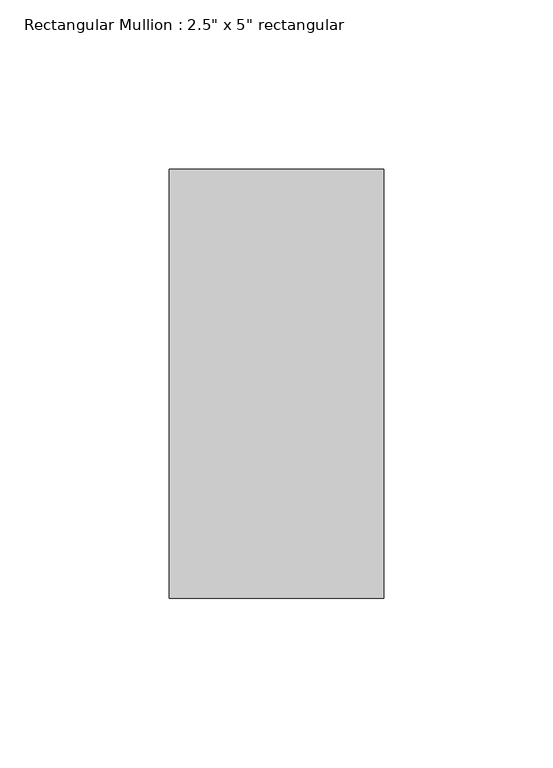
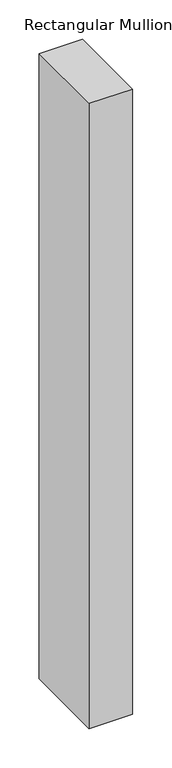
"""IFC4 building model written with IfcOpenShell, lengths in millimetres: member geometry."""

from ifc_helpers import new_model, si_unit, frame, origin, place, context, project, spatial, polyline, outline, extrude, source, transform, mapped, element, save


def member_43d3509f(model_context):
    return source(origin(), model_context, "Body", "SweptSolid", [
        extrude(outline(polyline([(0.0, 63.5), (0.0, -63.5), (-63.5, -63.5), (-63.5, 63.5), (0.0, 63.5)])), frame((0.0, 0.0, -969.4333333), z_axis=(0.0, 0.0, 1.0), x_axis=(1.0, 0.0, 0.0)), (0.0, 0.0, 1.0), 969.4333333),
    ])


if __name__ == "__main__":
    model = new_model("IFC4")
    model_context = context("Model", 3, world=origin())
    ifc_project = project(units=[si_unit("LENGTHUNIT", "METRE", prefix="MILLI")], contexts=[model_context])
    site = spatial("IfcSite", under=ifc_project)
    building = spatial("IfcBuilding", under=site)
    placement = place(None, origin())
    member_shape = member_43d3509f(model_context)
    element("IfcMember", 1, ObjectType="Rectangular Mullion : 2.5\" x 5\" rectangular", at=placement, inside=building, context=model_context, shape_type="MappedRepresentation", body=[
        mapped(member_shape, transform((0.0, 0.0, 0.0), x_axis=(1.0, 0.0, 0.0), y_axis=(0.0, 1.0, 0.0), z_axis=(0.0, 0.0, 1.0))),
    ])
    save(model, "model.ifc")

# Revit data of these elements
# Type "Rectangular Mullion : 2.5\" x 5\" rectangular"
#   built-in parameter 1007304 = 0.416667 (stored number, unit not read)
#   built-in parameter 1007301 = 0.104167 (stored number, unit not read)
#   built-in parameter 1007300 = 0.104167 (stored number, unit not read)
# Element 1 (IfcMember, "Rectangular Mullion : 2.5\" x 5\" rectangular")
#   Materials on its faces: "Aluminum"
# Materials
#   "Aluminum": class "Metal", colour RGB 247 247 247, transparency 0, Description = "Aluminum 6061", Cost = 0
